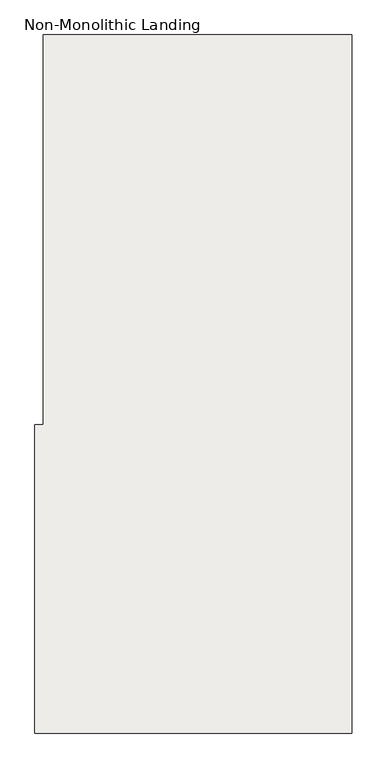
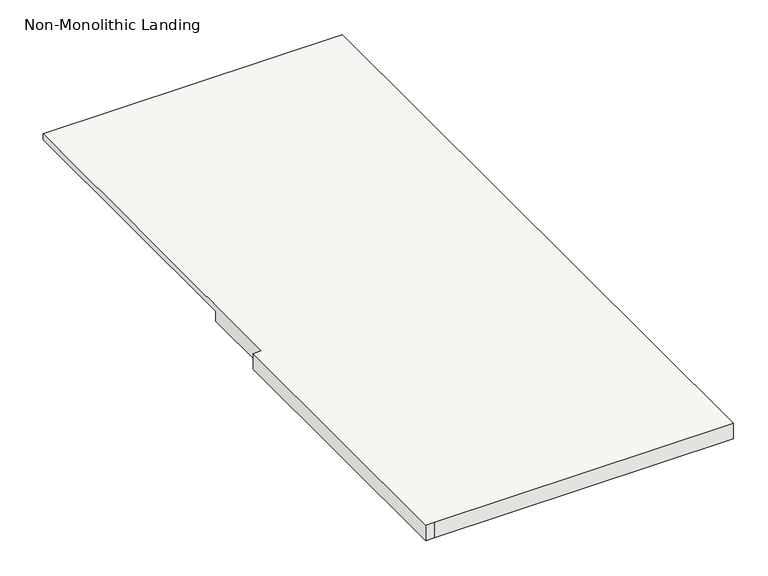
"""IFC4 building model written with IfcOpenShell, lengths in millimetres: slab geometry, Non-Monolithic Landing."""

from ifc_helpers import new_model, si_unit, origin, place, context, project, spatial, faceted_brep, source, transform, mapped, element, save


def non_monolithic_landing_dfce8634(model_context):
    return source(origin(), model_context, "Body", "Brep", [
        faceted_brep([(-2176.9017807, 1358.5428136, 4705.35), (-2151.5017807, 1358.5428136, 4679.95), (-2151.5017807, 444.1428136, 4679.95), (-2176.9017807, 444.1428136, 4705.35), (-2176.9017807, 202.2206867, 4724.4), (-2202.3017807, 202.2206867, 4724.4), (-2202.3017807, -712.1793133, 4724.4), (-2176.9017807, -712.1793133, 4724.4), (-1262.5017807, -712.1793133, 4724.4), (-1262.5017807, 1358.5428136, 4724.4), (-2176.9017807, 1358.5428136, 4724.4), (-2151.5017807, 444.1428136, 4673.6), (-2151.5017807, 1358.5428136, 4673.6), (-1262.5017807, 1358.5428136, 4673.6), (-1262.5017807, -712.1793133, 4673.6), (-2176.9017807, -712.1793133, 4673.6), (-2202.3017807, -712.1793133, 4673.6), (-2202.3017807, 202.2206867, 4673.6), (-2176.9017807, 202.2206867, 4673.6), (-2176.9017807, 444.1428136, 4673.6)], [[[0, 1, 2, 3]], [[4, 5, 6, 7, 8, 9, 10]], [[11, 12, 13, 14, 15, 16, 17, 18, 19]], [[12, 11, 2, 1]], [[11, 19, 3, 2]], [[4, 10, 0, 3, 19, 18]], [[5, 4, 18, 17]], [[6, 5, 17, 16]], [[7, 6, 16, 15]], [[8, 7, 15, 14]], [[9, 8, 14, 13]], [[10, 9, 13, 12, 1, 0]]]),
    ])


if __name__ == "__main__":
    model = new_model("IFC4")
    model_context = context("Model", 3, world=origin())
    ifc_project = project(units=[si_unit("LENGTHUNIT", "METRE", prefix="MILLI")], contexts=[model_context])
    site = spatial("IfcSite", under=ifc_project)
    building = spatial("IfcBuilding", under=site)
    placement = place(None, origin())
    non_monolithic_landing_shape = non_monolithic_landing_dfce8634(model_context)
    element("IfcSlab", 1, ObjectType="Non-Monolithic Landing", at=placement, inside=building, context=model_context, shape_type="MappedRepresentation", body=[
        mapped(non_monolithic_landing_shape, transform((0.0, 0.0, 0.0), x_axis=(1.0, 0.0, 0.0), y_axis=(0.0, 1.0, 0.0), z_axis=(0.0, 0.0, 1.0))),
    ])
    save(model, "model.ifc")
